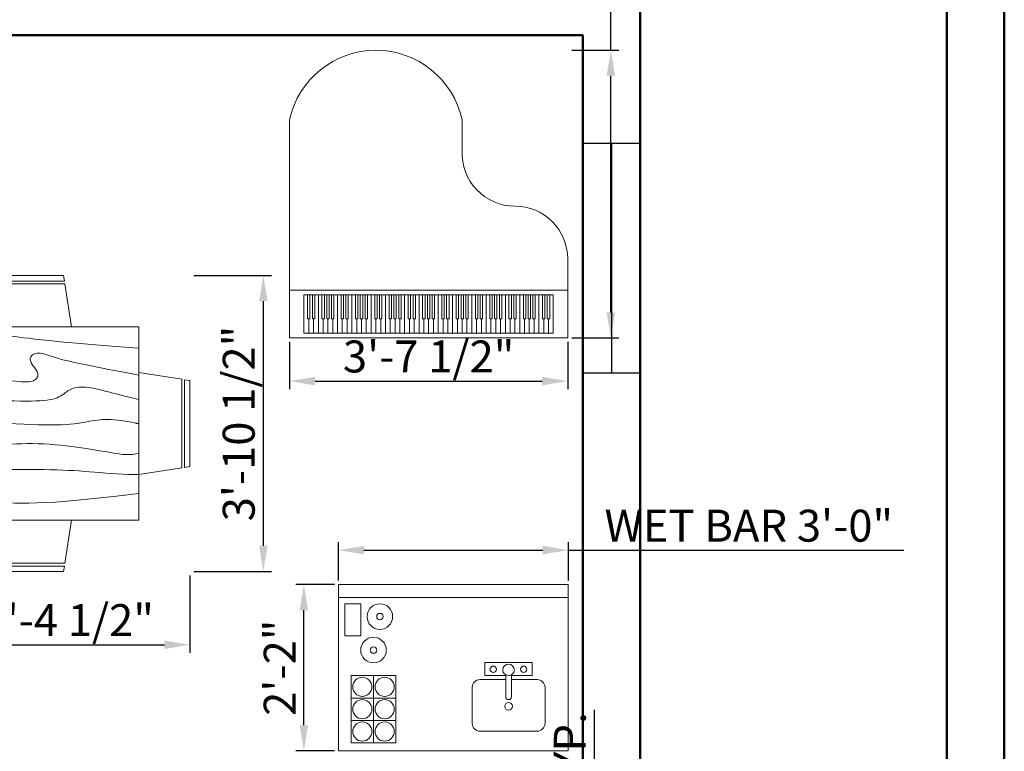
# Model space of a CAD drawing. Units: inches. Extents: x 116541 to 117938, y 135634 to 136328.
# Tile 8 of 9: x 117747 to 117902, y 135965 to 136080. Entities that reach past the tile are written whole.
import ezdxf

# ---------------------------------------------------------------- set-up
doc = ezdxf.new("R2010")
doc.units = ezdxf.units.IN
for name, color, linetype, lineweight in [('A-ANNO-DIMS', 2, 'Continuous', 18), ('A-FURN', 8, 'Continuous', 18), ('A-GLAZ', 1, 'Continuous', 25), ('A-WALL', 7, 'Continuous', 50)]:
    doc.layers.add(name, color=color, linetype=linetype, lineweight=lineweight)
doc.styles.get("Standard").update_dxf_attribs({"font": 'arial.ttf'})
doc.dimstyles.new('ISO-25', dxfattribs={"dimtxt": 5, "dimasz": 4, "dimexe": 1.25, "dimexo": 0.625, "dimtad": 1, "dimdec": 3, "dimlunit": 3, "dimtxsty": 'Standard', "dimcen": 2.5, "dimadec": 0, "dimazin": 0, "dimtfac": 1, "dimtdec": 3, "dimtmove": 0, "dimatfit": 3, "dimfxl": 1, "dimarcsym": 0})

# ---------------------------------------------------------------- blocks, each defined once
blk = doc.blocks.new('Dining Set - 36 x 72 in.')
for p, q in [((-22, 27.5), (-22.1562, 26.50042)), ((-22, 27.5), (-6, 27.5)), ((-5.8437, 26.49966), (-6, 27.5)), ((6, 27.5), (5.8438, 26.50042)), ((6, 27.5), (22, 27.5)), ((22.1563, 26.49966), (22, 27.5)), ((-22.2343, 26.00059), (-23.4847, 17.99762)), ((-22.2304, 26), (-5.7608, 26)), ((-5.8416, 26.5), (-22.1534, 26.5)), ((-4.5152, 17.99762), (-5.7655, 25.99926)), ((5.7657, 26.00059), (4.5153, 17.99762)), ((5.7696, 26), (22.2392, 26)), ((22.1584, 26.5), (5.8466, 26.5)), ((23.4848, 17.99762), (22.2345, 25.99926)), ((36, 18), (-36, 18)), ((-36, 18), (-36, -18)), ((36, -18), (36, 18)), ((-44.0006, 8.23428), (-35.9976, 9.48474)), ((44.0006, 8.23428), (35.9976, 9.48474)), ((-45.5, 8), (-44.5004, 8.15617)), ((-45.5, 8), (-45.5, -8)), ((-44.5, -8.15843), (-44.5, 8.15338)), ((-44, 8.23041), (-44, -8.23915)), ((44, 8.23041), (44, -8.23915)), ((44.5, -8.15843), (44.5, 8.15338)), ((45.5, 8), (44.5005, 8.15617)), ((45.5, 8), (45.5, -8)), ((-44.4997, -8.15631), (-45.5, -8)), ((-35.9976, -9.48476), (-43.9993, -8.2345)), ((35.9976, -9.48476), (43.9993, -8.2345)), ((44.4997, -8.15631), (45.5, -8)), ((-36, -18), (36, -18)), ((-22.2343, -26.0006), (-23.4847, -17.99762)), ((-4.5152, -17.99762), (-5.7655, -25.99928)), ((5.7657, -26.0006), (4.5153, -17.99762)), ((23.4848, -17.99762), (22.2345, -25.99928)), ((-22.2304, -26), (-5.7608, -26)), ((-22, -27.5), (-22.1562, -26.50044)), ((-5.8416, -26.5), (-22.1534, -26.5)), ((-5.8437, -26.49967), (-6, -27.5)), ((5.7696, -26), (22.2392, -26)), ((6, -27.5), (5.8438, -26.50044)), ((22.1584, -26.5), (5.8466, -26.5)), ((22.1563, -26.49967), (22, -27.5)), ((-22, -27.5), (-6, -27.5)), ((6, -27.5), (22, -27.5))]:
    blk.add_line(p, q)
for points in [[(-36, 15), (-31.1772, 14.97754), (-26.8079, 14.91406), (-22.8538, 14.81543), (-19.276, 14.6875), (-16.0362, 14.53613), (-13.0957, 14.36718), (-10.4159, 14.18652), (-7.9583, 14), (-5.6904, 13.81315), (-3.6035, 13.63021), (-1.6954, 13.45508), (0.0365, 13.29166), (1.5945, 13.14388), (2.9811, 13.01562), (4.1988, 12.9108), (5.25, 12.83333), (6.1393, 12.78613), (6.8802, 12.76823), (7.4883, 12.77767), (7.9792, 12.8125), (8.3685, 12.87077), (8.6719, 12.95052), (8.9049, 13.0498), (9.0833, 13.16666), (9.2205, 13.29899), (9.3216, 13.44401), (9.3895, 13.59879), (9.4271, 13.76041), (9.4373, 13.92594), (9.4232, 14.09245), (9.3875, 14.257), (9.3333, 14.41666), (9.2638, 14.56917), (9.1836, 14.71484), (9.0975, 14.85465), (9.0104, 14.98958), (8.9272, 15.1206), (8.8529, 15.2487), (8.7922, 15.37483), (8.75, 15.5), (8.7305, 15.62467), (8.7344, 15.74739), (8.7617, 15.86621), (8.8125, 15.97916), (8.8867, 16.08431), (8.9844, 16.17968), (9.1055, 16.26334), (9.25, 16.33333), (9.4189, 16.38802), (9.6172, 16.42708), (9.8506, 16.45052), (10.125, 16.45833), (10.4463, 16.45052), (10.8203, 16.42708), (11.2529, 16.38802), (11.75, 16.33333), (12.3184, 16.26318), (12.9694, 16.17838), (13.7151, 16.07991), (14.5677, 15.96875), (15.5395, 15.84586), (16.6426, 15.71224), (17.8893, 15.56884), (19.2917, 15.41666), (20.859, 15.25667), (22.5879, 15.08984), (24.4721, 14.91715), (26.5052, 14.73958), (28.6809, 14.5581), (30.9929, 14.3737), (33.4347, 14.18733), (36, 14)], [(-36, 10), (-28.9766, 10.14274), (-23.1725, 10.20442), (-18.4241, 10.19775), (-14.5677, 10.13541), (-11.4399, 10.03011), (-8.877, 9.89453), (-6.7154, 9.74137), (-4.7917, 9.58333), (-2.9698, 9.43082), (-1.2246, 9.28515), (0.4415, 9.14534), (2.026, 9.01041), (3.5266, 8.87939), (4.9408, 8.7513), (6.266, 8.62516), (7.5, 8.5), (8.6411, 8.37549), (9.6914, 8.2539), (10.6538, 8.13818), (11.5312, 8.03125), (12.3267, 7.93603), (13.043, 7.85547), (13.6831, 7.79248), (14.25, 7.75), (14.7471, 7.7303), (15.1797, 7.73307), (15.5537, 7.75732), (15.875, 7.80208), (16.1494, 7.86637), (16.3828, 7.94922), (16.5811, 8.04964), (16.75, 8.16666), (16.8944, 8.29915), (17.0143, 8.44531), (17.1089, 8.60319), (17.1771, 8.77083), (17.218, 8.94629), (17.2305, 9.1276), (17.2137, 9.31282), (17.1667, 9.5), (17.0895, 9.6875), (16.987, 9.875), (16.8649, 10.0625), (16.7292, 10.25), (16.5856, 10.4375), (16.4401, 10.625), (16.2985, 10.8125), (16.1667, 11), (16.05, 11.18733), (15.9518, 11.3737), (15.8752, 11.5581), (15.8229, 11.73958), (15.798, 11.91715), (15.8034, 12.08984), (15.842, 12.25667), (15.9167, 12.41666), (16.0295, 12.56836), (16.1784, 12.70833), (16.3605, 12.83268), (16.5729, 12.9375), (16.8127, 13.01888), (17.0768, 13.07291), (17.3625, 13.0957), (17.6667, 13.08333), (17.9894, 13.03312), (18.3418, 12.94726), (18.7382, 12.82918), (19.1927, 12.68229), (19.7195, 12.51001), (20.3327, 12.31575), (21.0465, 12.10294), (21.875, 11.875), (22.8357, 11.63354), (23.959, 11.37304), (25.2786, 11.08618), (26.8282, 10.76562), (28.6414, 10.40405), (30.752, 9.99414), (33.1936, 9.52856), (36, 9)], [(-36, 5.5), (-30.7157, 5.3348), (-26.069, 5.20963), (-21.9946, 5.11767), (-18.4271, 5.05208), (-15.3009, 5.00602), (-12.5508, 4.97265), (-10.1112, 4.94515), (-7.9167, 4.91666), (-5.909, 4.88167), (-4.0586, 4.83984), (-2.3429, 4.79215), (-0.7396, 4.73958), (0.7739, 4.6831), (2.22, 4.6237), (3.6213, 4.56233), (5, 4.5), (6.373, 4.43782), (7.7344, 4.3776), (9.0723, 4.32129), (10.375, 4.27083), (11.6309, 4.22819), (12.8281, 4.19531), (13.9551, 4.17415), (15, 4.16666), (15.954, 4.17448), (16.819, 4.19791), (17.6001, 4.23698), (18.3021, 4.29166), (18.9299, 4.36198), (19.4883, 4.44791), (19.9823, 4.54948), (20.4167, 4.66666), (20.7969, 4.79899), (21.1302, 4.94401), (21.4245, 5.09879), (21.6875, 5.26041), (21.9271, 5.42594), (22.1511, 5.59245), (22.3672, 5.757), (22.5834, 5.91666), (22.8065, 6.06868), (23.0404, 6.21093), (23.2879, 6.34147), (23.5521, 6.45833), (23.8358, 6.55957), (24.142, 6.64323), (24.4735, 6.70735), (24.8334, 6.75), (25.2235, 6.76969), (25.642, 6.76692), (26.0858, 6.74267), (26.5521, 6.69791), (27.0379, 6.63362), (27.5404, 6.55078), (28.0565, 6.45036), (28.5834, 6.33333), (29.1242, 6.19987), (29.7071, 6.04687), (30.3661, 5.87044), (31.1354, 5.66666), (32.0493, 5.43164), (33.142, 5.16146), (34.4475, 4.85221), (36, 4.5)], [(-36, -1), (-30.7915, -0.6591), (-26.0195, -0.38216), (-21.6519, -0.16284), (-17.6563, 0.00521), (-14.0005, 0.12833), (-10.6523, 0.21289), (-7.5796, 0.26522), (-4.75, 0.29166), (-2.134, 0.29793), (0.2878, 0.28711), (2.5317, 0.26163), (4.6146, 0.22396), (6.5529, 0.17651), (8.3633, 0.12174), (10.0623, 0.06209), (11.6667, 0), (13.1899, -0.06201), (14.6341, -0.1211), (15.9982, -0.17432), (17.2813, -0.21875), (18.4823, -0.25147), (19.6003, -0.26953), (20.6343, -0.27002), (21.5834, -0.25), (22.4481, -0.20768), (23.2357, -0.14584), (23.9549, -0.06836), (24.6146, 0.02083), (25.2235, 0.11784), (25.7904, 0.21875), (26.3241, 0.31966), (26.8334, 0.41666), (27.3265, 0.50618), (27.8099, 0.58593), (28.2894, 0.65397), (28.7709, 0.70833), (29.2601, 0.74707), (29.763, 0.76823), (30.2855, 0.76985), (30.8334, 0.75), (31.4088, 0.70784), (31.9994, 0.64713), (32.589, 0.57275), (33.1615, 0.48958), (33.7008, 0.4025), (34.1908, 0.3164), (34.6153, 0.23616), (34.9584, 0.16666), (35.2099, 0.11165), (35.3848, 0.07031), (35.504, 0.04069), (35.5886, 0.02083), (35.6594, 0.00879), (35.7377, 0.0026), (35.8442, 0.00032), (36, 0)], [(-36, -6.5), (-27.1843, -6.31267), (-20.084, -6.1263), (-14.469, -5.9419), (-10.1094, -5.76042), (-6.7752, -5.58285), (-4.2363, -5.41016), (-2.2629, -5.24333), (-0.625, -5.08334), (0.8708, -4.93099), (2.2715, -4.78646), (3.5872, -4.64974), (4.8281, -4.52084), (6.0046, -4.39974), (7.127, -4.28646), (8.2053, -4.18099), (9.25, -4.08334), (10.2705, -3.99382), (11.2734, -3.91407), (12.2647, -3.84603), (13.25, -3.79167), (14.2354, -3.75293), (15.2266, -3.73177), (16.2295, -3.73015), (17.25, -3.75), (18.2912, -3.79248), (19.3451, -3.85547), (20.4009, -3.93604), (21.4479, -4.03125), (22.4754, -4.13819), (23.4727, -4.25391), (24.4289, -4.37549), (25.3334, -4.5), (26.1785, -4.62492), (26.9694, -4.74935), (27.7145, -4.87281), (28.4219, -4.99479), (29.1, -5.11483), (29.7572, -5.23242), (30.4016, -5.34709), (31.0417, -5.45834), (31.6837, -5.56437), (32.3262, -5.65821), (32.9658, -5.73153), (33.599, -5.77604), (34.2224, -5.78345), (34.8327, -5.74545), (35.4264, -5.65373), (36, -5.5)], [(-36, -10), (-26.4022, -9.81299), (-18.4675, -9.62891), (-11.9839, -9.45069), (-6.7396, -9.28125), (-2.5226, -9.12354), (0.8789, -8.98047), (3.6769, -8.85498), (6.0833, -8.75), (8.2767, -8.66765), (10.3021, -8.60677), (12.1712, -8.56543), (13.8958, -8.54167), (15.4876, -8.53353), (16.9583, -8.53907), (18.3197, -8.55632), (19.5834, -8.58334), (20.7616, -8.61841), (21.8685, -8.66081), (22.9188, -8.71004), (23.9271, -8.76563), (24.9081, -8.82707), (25.8763, -8.89388), (26.8465, -8.96558), (27.8334, -9.04167), (28.8474, -9.12118), (29.8828, -9.20117), (30.93, -9.27824), (31.9792, -9.34896), (33.0205, -9.40991), (34.0443, -9.45768), (35.0407, -9.48885), (36, -9.5)], [(-36, -14.5), (-30.0881, -14.33513), (-25.0332, -14.21224), (-20.7312, -14.12647), (-17.0781, -14.07292), (-13.97, -14.04671), (-11.3027, -14.04297), (-8.9724, -14.05681), (-6.875, -14.08334), (-4.9224, -14.11833), (-3.0905, -14.16016), (-1.3709, -14.20785), (0.2448, -14.26042), (1.7647, -14.3169), (3.1973, -14.3763), (4.5507, -14.43767), (5.8333, -14.5), (7.0554, -14.5621), (8.235, -14.62175), (9.3922, -14.67652), (10.5469, -14.72396), (11.7192, -14.76164), (12.929, -14.78711), (14.1965, -14.79794), (15.5417, -14.79167), (16.9933, -14.76424), (18.6152, -14.70508), (20.4804, -14.60197), (22.6615, -14.44271), (25.2312, -14.21509), (28.2624, -13.9069), (31.8277, -13.50594), (36, -13)]]:
    blk.add_lwpolyline(points)
blk = doc.blocks.new('Piano - Baby Grand')
for p, q in [((-29, 8.250005), (-29, -27.249995)), ((7, 1.250005), (7, 8.250005)), ((29, -20.749995), (29, -27.249995)), ((-29, -27.249995), (-29, -37.249995)), ((29, -27.249995), (-29, -27.249995)), ((-26, -36.249995), (-26, -28.249995)), ((-26, -28.249995), (26, -28.249995)), ((-25.25, -33.249995), (-25.25, -28.249995)), ((-24.75, -28.249995), (-24.75, -33.249995)), ((-24.25, -33.249995), (-24.25, -28.249995)), ((-23.75, -28.249995), (-23.75, -33.249995)), ((-23, -36.249995), (-23, -28.249995)), ((-22.25, -33.249995), (-22.25, -28.249995)), ((-21.75, -28.249995), (-21.75, -33.249995)), ((-21.25, -33.249995), (-21.25, -28.249995)), ((-20.75, -28.249995), (-20.75, -33.249995)), ((-20.25, -33.249995), (-20.25, -28.249995)), ((-19.75, -28.249995), (-19.75, -33.249995)), ((-19, -36.249995), (-19, -28.249995)), ((-18.25, -33.249995), (-18.25, -28.249995)), ((-17.75, -28.249995), (-17.75, -33.249995)), ((-17.25, -33.249995), (-17.25, -28.249995)), ((-16.75, -28.249995), (-16.75, -33.249995)), ((-16, -36.249995), (-16, -28.249995)), ((-15.25, -33.249995), (-15.25, -28.249995)), ((-14.75, -28.249995), (-14.75, -33.249995)), ((-14.25, -33.249995), (-14.25, -28.249995)), ((-13.75, -28.249995), (-13.75, -33.249995)), ((-13.25, -33.249995), (-13.25, -28.249995)), ((-12.75, -28.249995), (-12.75, -33.249995)), ((-12, -36.249995), (-12, -28.249995)), ((-11.25, -33.249995), (-11.25, -28.249995)), ((-10.75, -28.249995), (-10.75, -33.249995)), ((-10.25, -33.249995), (-10.25, -28.249995)), ((-9.75, -28.249995), (-9.75, -33.249995)), ((-9, -36.249995), (-9, -28.249995)), ((-8.25, -33.249995), (-8.25, -28.249995)), ((-7.75, -28.249995), (-7.75, -33.249995)), ((-7.25, -33.249995), (-7.25, -28.249995)), ((-6.75, -28.249995), (-6.75, -33.249995)), ((-6.25, -33.249995), (-6.25, -28.249995)), ((-5.75, -28.249995), (-5.75, -33.249995)), ((-5, -36.249995), (-5, -28.249995)), ((-4.25, -33.249995), (-4.25, -28.249995)), ((-3.75, -28.249995), (-3.75, -33.249995)), ((-3.25, -33.249995), (-3.25, -28.249995)), ((-2.75, -28.249995), (-2.75, -33.249995)), ((-2, -36.249995), (-2, -28.249995)), ((-1.25, -33.249995), (-1.25, -28.249995)), ((-0.75, -28.249995), (-0.75, -33.249995)), ((-0.25, -33.249995), (-0.25, -28.249995)), ((0.25, -28.249995), (0.25, -33.249995)), ((0.75, -33.249995), (0.75, -28.249995)), ((1.25, -28.249995), (1.25, -33.249995)), ((2, -36.249995), (2, -28.249995)), ((2.75, -33.249995), (2.75, -28.249995)), ((3.25, -28.249995), (3.25, -33.249995)), ((3.75, -33.249995), (3.75, -28.249995)), ((4.25, -28.249995), (4.25, -33.249995)), ((5, -36.249995), (5, -28.249995)), ((5.75, -33.249995), (5.75, -28.249995)), ((6.25, -28.249995), (6.25, -33.249995)), ((6.75, -33.249995), (6.75, -28.249995)), ((7.25, -28.249995), (7.25, -33.249995)), ((7.75, -33.249995), (7.75, -28.249995)), ((8.25, -28.249995), (8.25, -33.249995)), ((9, -36.249995), (9, -28.249995)), ((9.75, -33.249995), (9.75, -28.249995)), ((10.25, -28.249995), (10.25, -33.249995)), ((10.75, -33.249995), (10.75, -28.249995)), ((11.25, -28.249995), (11.25, -33.249995)), ((12, -36.249995), (12, -28.249995)), ((12.75, -33.249995), (12.75, -28.249995)), ((13.25, -28.249995), (13.25, -33.249995)), ((13.75, -33.249995), (13.75, -28.249995)), ((14.25, -28.249995), (14.25, -33.249995)), ((14.75, -33.249995), (14.75, -28.249995)), ((15.25, -28.249995), (15.25, -33.249995)), ((16, -36.249995), (16, -28.249995)), ((16.75, -33.249995), (16.75, -28.249995)), ((17.25, -28.249995), (17.25, -33.249995)), ((17.75, -33.249995), (17.75, -28.249995)), ((18.25, -28.249995), (18.25, -33.249995)), ((19, -36.249995), (19, -28.249995)), ((19.75, -33.249995), (19.75, -28.249995)), ((20.25, -28.249995), (20.25, -33.249995)), ((20.75, -33.249995), (20.75, -28.249995)), ((21.25, -28.249995), (21.25, -33.249995)), ((21.75, -33.249995), (21.75, -28.249995)), ((22.25, -28.249995), (22.25, -33.249995)), ((23, -36.249995), (23, -28.249995)), ((23.75, -33.249995), (23.75, -28.249995)), ((24.25, -28.249995), (24.25, -33.249995)), ((24.75, -33.249995), (24.75, -28.249995)), ((25.25, -28.249995), (25.25, -33.249995)), ((26, -36.249995), (26, -28.249995)), ((29, -37.249995), (29, -27.249995)), ((-25, -33.249995), (-25.25, -33.249995)), ((-24.75, -33.249995), (-25, -33.249995)), ((-25, -36.249995), (-25, -33.249995)), ((-24, -33.249995), (-24.25, -33.249995)), ((-23.75, -33.249995), (-24, -33.249995)), ((-24, -36.249995), (-24, -33.249995)), ((-22, -33.249995), (-22.25, -33.249995)), ((-21.75, -33.249995), (-22, -33.249995)), ((-22, -36.249995), (-22, -33.249995)), ((-21, -33.249995), (-21.25, -33.249995)), ((-20.75, -33.249995), (-21, -33.249995)), ((-21, -36.249995), (-21, -33.249995)), ((-20, -33.249995), (-20.25, -33.249995)), ((-19.75, -33.249995), (-20, -33.249995)), ((-20, -36.249995), (-20, -33.249995)), ((-18, -33.249995), (-18.25, -33.249995)), ((-17.75, -33.249995), (-18, -33.249995)), ((-18, -36.249995), (-18, -33.249995)), ((-17, -33.249995), (-17.25, -33.249995)), ((-16.75, -33.249995), (-17, -33.249995)), ((-17, -36.249995), (-17, -33.249995)), ((-15, -33.249995), (-15.25, -33.249995)), ((-14.75, -33.249995), (-15, -33.249995)), ((-15, -36.249995), (-15, -33.249995)), ((-14, -33.249995), (-14.25, -33.249995)), ((-13.75, -33.249995), (-14, -33.249995)), ((-14, -36.249995), (-14, -33.249995)), ((-13, -33.249995), (-13.25, -33.249995)), ((-12.75, -33.249995), (-13, -33.249995)), ((-13, -36.249995), (-13, -33.249995)), ((-11, -33.249995), (-11.25, -33.249995)), ((-10.75, -33.249995), (-11, -33.249995)), ((-11, -36.249995), (-11, -33.249995)), ((-10, -33.249995), (-10.25, -33.249995)), ((-9.75, -33.249995), (-10, -33.249995)), ((-10, -36.249995), (-10, -33.249995)), ((-8, -33.249995), (-8.25, -33.249995)), ((-7.75, -33.249995), (-8, -33.249995)), ((-8, -36.249995), (-8, -33.249995)), ((-7, -33.249995), (-7.25, -33.249995)), ((-6.75, -33.249995), (-7, -33.249995)), ((-7, -36.249995), (-7, -33.249995)), ((-6, -33.249995), (-6.25, -33.249995)), ((-5.75, -33.249995), (-6, -33.249995)), ((-6, -36.249995), (-6, -33.249995)), ((-4, -33.249995), (-4.25, -33.249995)), ((-3.75, -33.249995), (-4, -33.249995)), ((-4, -36.249995), (-4, -33.249995)), ((-3, -33.249995), (-3.25, -33.249995)), ((-2.75, -33.249995), (-3, -33.249995)), ((-3, -36.249995), (-3, -33.249995)), ((-1, -33.249995), (-1.25, -33.249995)), ((-0.75, -33.249995), (-1, -33.249995)), ((-1, -36.249995), (-1, -33.249995)), ((0, -33.249995), (-0.25, -33.249995)), ((0.25, -33.249995), (0, -33.249995)), ((0, -36.249995), (0, -33.249995)), ((1, -33.249995), (0.75, -33.249995)), ((1.25, -33.249995), (1, -33.249995)), ((1, -36.249995), (1, -33.249995)), ((3, -33.249995), (2.75, -33.249995)), ((3.25, -33.249995), (3, -33.249995)), ((3, -36.249995), (3, -33.249995)), ((4, -33.249995), (3.75, -33.249995)), ((4.25, -33.249995), (4, -33.249995)), ((4, -36.249995), (4, -33.249995)), ((6, -33.249995), (5.75, -33.249995)), ((6.25, -33.249995), (6, -33.249995)), ((6, -36.249995), (6, -33.249995)), ((7, -33.249995), (6.75, -33.249995)), ((7.25, -33.249995), (7, -33.249995)), ((7, -36.249995), (7, -33.249995)), ((8, -33.249995), (7.75, -33.249995)), ((8.25, -33.249995), (8, -33.249995)), ((8, -36.249995), (8, -33.249995)), ((10, -33.249995), (9.75, -33.249995)), ((10.25, -33.249995), (10, -33.249995)), ((10, -36.249995), (10, -33.249995)), ((11, -33.249995), (10.75, -33.249995)), ((11.25, -33.249995), (11, -33.249995)), ((11, -36.249995), (11, -33.249995)), ((13, -33.249995), (12.75, -33.249995)), ((13.25, -33.249995), (13, -33.249995)), ((13, -36.249995), (13, -33.249995)), ((14, -33.249995), (13.75, -33.249995)), ((14.25, -33.249995), (14, -33.249995)), ((14, -36.249995), (14, -33.249995)), ((15, -33.249995), (14.75, -33.249995)), ((15.25, -33.249995), (15, -33.249995)), ((15, -36.249995), (15, -33.249995)), ((17, -33.249995), (16.75, -33.249995)), ((17.25, -33.249995), (17, -33.249995)), ((17, -36.249995), (17, -33.249995)), ((18, -33.249995), (17.75, -33.249995)), ((18.25, -33.249995), (18, -33.249995)), ((18, -36.249995), (18, -33.249995)), ((20, -33.249995), (19.75, -33.249995)), ((20.25, -33.249995), (20, -33.249995)), ((20, -36.249995), (20, -33.249995)), ((21, -33.249995), (20.75, -33.249995)), ((21.25, -33.249995), (21, -33.249995)), ((21, -36.249995), (21, -33.249995)), ((22, -33.249995), (21.75, -33.249995)), ((22.25, -33.249995), (22, -33.249995)), ((22, -36.249995), (22, -33.249995)), ((24, -33.249995), (23.75, -33.249995)), ((24.25, -33.249995), (24, -33.249995)), ((24, -36.249995), (24, -33.249995)), ((25, -33.249995), (24.75, -33.249995)), ((25.25, -33.249995), (25, -33.249995)), ((25, -36.249995), (25, -33.249995)), ((-26, -36.249995), (-25, -36.249995)), ((-25, -36.249995), (-24, -36.249995)), ((-24, -36.249995), (-23, -36.249995)), ((-23, -36.249995), (-22, -36.249995)), ((-22, -36.249995), (-21, -36.249995)), ((-21, -36.249995), (-20, -36.249995)), ((-20, -36.249995), (-19, -36.249995)), ((-19, -36.249995), (-18, -36.249995)), ((-18, -36.249995), (-17, -36.249995)), ((-17, -36.249995), (-16, -36.249995)), ((-16, -36.249995), (-15, -36.249995)), ((-15, -36.249995), (-14, -36.249995)), ((-14, -36.249995), (-13, -36.249995)), ((-13, -36.249995), (-12, -36.249995)), ((-12, -36.249995), (-11, -36.249995)), ((-11, -36.249995), (-10, -36.249995)), ((-10, -36.249995), (-9, -36.249995)), ((-9, -36.249995), (-8, -36.249995)), ((-8, -36.249995), (-7, -36.249995)), ((-7, -36.249995), (-6, -36.249995)), ((-6, -36.249995), (-5, -36.249995)), ((-5, -36.249995), (-4, -36.249995)), ((-4, -36.249995), (-3, -36.249995)), ((-3, -36.249995), (-2, -36.249995)), ((-2, -36.249995), (-1, -36.249995)), ((-1, -36.249995), (0, -36.249995)), ((0, -36.249995), (1, -36.249995)), ((1, -36.249995), (2, -36.249995)), ((2, -36.249995), (3, -36.249995)), ((3, -36.249995), (4, -36.249995)), ((4, -36.249995), (5, -36.249995)), ((5, -36.249995), (6, -36.249995)), ((6, -36.249995), (7, -36.249995)), ((7, -36.249995), (8, -36.249995)), ((8, -36.249995), (9, -36.249995)), ((9, -36.249995), (10, -36.249995)), ((10, -36.249995), (11, -36.249995)), ((11, -36.249995), (12, -36.249995)), ((12, -36.249995), (13, -36.249995)), ((13, -36.249995), (14, -36.249995)), ((14, -36.249995), (15, -36.249995)), ((15, -36.249995), (16, -36.249995)), ((16, -36.249995), (17, -36.249995)), ((17, -36.249995), (18, -36.249995)), ((18, -36.249995), (19, -36.249995)), ((19, -36.249995), (20, -36.249995)), ((20, -36.249995), (21, -36.249995)), ((21, -36.249995), (22, -36.249995)), ((22, -36.249995), (23, -36.249995)), ((23, -36.249995), (24, -36.249995)), ((24, -36.249995), (25, -36.249995)), ((25, -36.249995), (26, -36.249995)), ((-29, -37.249995), (29, -37.249995))]:
    blk.add_line(p, q)
for centre, radius, start, end in [((-11, 4.327585), 18.42241, 12.29325, 167.7067), ((18, 1.250005), 11, 177.3974, 270), ((18, -20.749995), 11, 0, 90)]:
    blk.add_arc(centre, radius, start, end)
blk = doc.blocks.new('Wet Bar')
for p, q in [((0, 0), (36, 0)), ((0, -26), (0, 0)), ((36, 0), (36, -26)), ((0, -2), (36, -2)), ((3.5, -3), (1, -3)), ((1, -3), (1, -8)), ((3.5, -8), (3.5, -3)), ((1, -8), (3.5, -8)), ((2, -14.25), (9, -14.25)), ((2, -24.75), (2, -14.25)), ((5.5, -14.25), (5.5, -24.75)), ((9, -14.25), (9, -24.75)), ((26.2, -17.55), (26.2, -14.1284)), ((27.1001, -17.55), (27.1001, -14.1284)), ((2, -17.75), (9, -17.75)), ((9, -21.25), (2, -21.25)), ((36, -26), (0, -26)), ((9, -24.75), (2, -24.75))]:
    blk.add_line(p, q)
for points in [[(26.2, -14.25), (22.95, -14.25), (22.95, -12.2), (26.75, -12.2)], [(26.7487, -12.2), (30.3501, -12.2), (30.3501, -14.25), (27.1001, -14.25)], [(22.15, -14.85), (26.2, -14.85)], [(27.1001, -14.85), (31.15, -14.85)], [(20.95, -21.75), (20.95, -16.05)], [(32.3501, -16.05), (32.3501, -21.75)], [(31.15, -22.95), (22.15, -22.95)]]:
    blk.add_lwpolyline(points)
for centre, radius in [((6.5, -5), 2), ((6.5, -5), 0.5), ((5.5, -10.25), 2), ((5.5, -10.25), 0.5), ((24.25, -13.25), 0.5), ((26.65, -13.35), 0.9), ((29, -13.25), 0.5), ((3.75, -16), 1.5), ((7.25, -16), 1.5), ((3.75, -19.5), 1.5), ((7.25, -19.5), 1.5), ((26.65, -19.05), 0.6), ((3.75, -23), 1.5), ((7.25, -23), 1.5)]:
    blk.add_circle(centre, radius)
for centre, radius, start, end in [((22.2251, -16.125), 1.2772, 93.36646, 176.6335), ((31.075, -16.125), 1.2772, 3.366461, 86.63354), ((26.65, -17.55), 0.45, 180, 0), ((22.2251, -21.675), 1.2772, 183.3665, 266.6335), ((31.075, -21.675), 1.2772, 273.3665, 356.6335)]:
    blk.add_arc(centre, radius, start, end)
blk = doc.blocks.new('*D61')
at = {"layer": 'A-ANNO-DIMS', "color": 0, "lineweight": -2, "transparency": 16777216}
for p, q in [((117837.36, 135924.99), (117837.36, 135971.9)), ((117835.14, 135924.99), (117838.61, 135924.99)), ((117837.36, 135913.66), (117837.36, 135920.99)), ((117835.14, 135909.66), (117838.61, 135909.66))]:
    blk.add_line(p, q, dxfattribs=at)
at = {"layer": 'A-ANNO-DIMS', "color": 0, "transparency": 16777216}
for points in [[(117836.7, 135920.99), (117838.03, 135920.99), (117837.36, 135924.99)], [(117836.7, 135913.66), (117838.03, 135913.66), (117837.36, 135909.66)]]:
    blk.add_solid(points, dxfattribs=at)
at = {"layer": 'Defpoints', "color": 0, "transparency": 16777216}
for p in [(117834.51, 135924.99), (117837.36, 135924.99), (117834.51, 135909.66)]:
    blk.add_point(p, dxfattribs=at)
at = {"layer": 'A-ANNO-DIMS', "color": 0, "transparency": 16777216, "insert": (117834.15, 135950.44), "char_height": 5, "attachment_point": 5, "rotation": 90}
blk.add_mtext('1\'-3 1/2" TYP.', dxfattribs=at)
blk = doc.blocks.new('*D80')
at = {"layer": 'A-ANNO-DIMS', "color": 0, "lineweight": -2, "transparency": 16777216}
for p, q in [((117697.46, 135992.95), (117697.46, 135980.84)), ((117774.05, 135992.95), (117774.05, 135980.84)), ((117701.46, 135982.09), (117770.05, 135982.09))]:
    blk.add_line(p, q, dxfattribs=at)
at = {"layer": 'A-ANNO-DIMS', "color": 0, "transparency": 16777216}
for points in [[(117701.46, 135982.75), (117701.46, 135981.42), (117697.46, 135982.09)], [(117770.05, 135982.75), (117770.05, 135981.42), (117774.05, 135982.09)]]:
    blk.add_solid(points, dxfattribs=at)
at = {"layer": 'Defpoints', "color": 0, "transparency": 16777216}
for p in [(117697.46, 135993.58), (117774.05, 135993.58), (117774.05, 135982.09)]:
    blk.add_point(p, dxfattribs=at)
at = {"layer": 'A-ANNO-DIMS', "color": 0, "transparency": 16777216, "insert": (117735.75, 135985.3), "char_height": 5, "attachment_point": 5}
blk.add_mtext('DINING SET 6\'-4 1/2"', dxfattribs=at)
blk = doc.blocks.new('*D81')
at = {"layer": 'A-ANNO-DIMS', "color": 0, "lineweight": -2, "transparency": 16777216}
for p, q in [((117774.67, 136039.87), (117786.79, 136039.87)), ((117785.54, 135997.58), (117785.54, 136035.87)), ((117774.67, 135993.58), (117786.79, 135993.58))]:
    blk.add_line(p, q, dxfattribs=at)
at = {"layer": 'A-ANNO-DIMS', "color": 0, "transparency": 16777216}
for points in [[(117784.87, 136035.87), (117786.2, 136035.87), (117785.54, 136039.87)], [(117784.87, 135997.58), (117786.2, 135997.58), (117785.54, 135993.58)]]:
    blk.add_solid(points, dxfattribs=at)
at = {"layer": 'Defpoints', "color": 0, "transparency": 16777216}
for p in [(117774.05, 136039.87), (117785.54, 136039.87), (117774.05, 135993.58)]:
    blk.add_point(p, dxfattribs=at)
at = {"layer": 'A-ANNO-DIMS', "color": 0, "transparency": 16777216, "insert": (117782.33, 136016.72), "char_height": 5, "attachment_point": 5, "rotation": 90}
blk.add_mtext('3\'-10 1/2"', dxfattribs=at)
blk = doc.blocks.new('*D96')
at = {"layer": 'A-ANNO-DIMS', "color": 0, "lineweight": -2, "transparency": 16777216}
for p, q in [((117839.93, 136075.15), (117839.93, 136164.88)), ((117833.8, 136075.15), (117841.18, 136075.15)), ((117839.93, 136034.11), (117839.93, 136071.15)), ((117833.8, 136030.11), (117841.18, 136030.11))]:
    blk.add_line(p, q, dxfattribs=at)
at = {"layer": 'A-ANNO-DIMS', "color": 0, "transparency": 16777216}
for points in [[(117839.26, 136071.15), (117840.6, 136071.15), (117839.93, 136075.15)], [(117839.26, 136034.11), (117840.6, 136034.11), (117839.93, 136030.11)]]:
    blk.add_solid(points, dxfattribs=at)
at = {"layer": 'Defpoints', "color": 0, "transparency": 16777216}
for p in [(117833.18, 136075.15), (117839.93, 136075.15), (117833.18, 136030.11)]:
    blk.add_point(p, dxfattribs=at)
at = {"layer": 'A-ANNO-DIMS', "color": 0, "transparency": 16777216, "insert": (117836.72, 136122.01), "char_height": 5, "attachment_point": 5, "rotation": 90}
blk.add_mtext('BABY GRAND PIANO 3\'-9"', dxfattribs=at)
blk = doc.blocks.new('*D97')
at = {"layer": 'A-ANNO-DIMS', "color": 0, "lineweight": -2, "transparency": 16777216}
for p, q in [((117789.64, 136029.49), (117789.64, 136022.11)), ((117833.18, 136029.49), (117833.18, 136022.11)), ((117793.64, 136023.36), (117829.18, 136023.36))]:
    blk.add_line(p, q, dxfattribs=at)
at = {"layer": 'A-ANNO-DIMS', "color": 0, "transparency": 16777216}
for points in [[(117793.64, 136024.02), (117793.64, 136022.69), (117789.64, 136023.36)], [(117829.18, 136024.02), (117829.18, 136022.69), (117833.18, 136023.36)]]:
    blk.add_solid(points, dxfattribs=at)
at = {"layer": 'Defpoints', "color": 0, "transparency": 16777216}
for p in [(117789.64, 136030.11), (117833.18, 136030.11), (117833.18, 136023.36)]:
    blk.add_point(p, dxfattribs=at)
at = {"layer": 'A-ANNO-DIMS', "color": 0, "transparency": 16777216, "insert": (117811.41, 136026.57), "char_height": 5, "attachment_point": 5}
blk.add_mtext('3\'-7 1/2"', dxfattribs=at)
blk = doc.blocks.new('*D98')
at = {"layer": 'A-ANNO-DIMS', "color": 0, "lineweight": -2, "transparency": 16777216}
for p, q in [((117797.28, 135992.13), (117797.28, 135998.15)), ((117833.28, 135992.13), (117833.28, 135998.15)), ((117801.28, 135996.9), (117829.28, 135996.9)), ((117833.28, 135996.9), (117885.78, 135996.9))]:
    blk.add_line(p, q, dxfattribs=at)
at = {"layer": 'A-ANNO-DIMS', "color": 0, "transparency": 16777216}
for points in [[(117801.28, 135997.57), (117801.28, 135996.24), (117797.28, 135996.9)], [(117829.28, 135997.57), (117829.28, 135996.24), (117833.28, 135996.9)]]:
    blk.add_solid(points, dxfattribs=at)
at = {"layer": 'Defpoints', "color": 0, "transparency": 16777216}
for p in [(117833.28, 135996.9), (117797.28, 135991.5), (117833.28, 135991.5)]:
    blk.add_point(p, dxfattribs=at)
at = {"layer": 'A-ANNO-DIMS', "color": 0, "transparency": 16777216, "insert": (117861.53, 136000.08), "char_height": 5, "attachment_point": 5}
blk.add_mtext('WET BAR 3\'-0"', dxfattribs=at)
blk = doc.blocks.new('*D99')
at = {"layer": 'A-ANNO-DIMS', "color": 0, "lineweight": -2, "transparency": 16777216}
for p, q in [((117796.65, 135991.5), (117790.63, 135991.5)), ((117791.88, 135969.5), (117791.88, 135987.5)), ((117796.65, 135965.5), (117790.63, 135965.5))]:
    blk.add_line(p, q, dxfattribs=at)
at = {"layer": 'A-ANNO-DIMS', "color": 0, "transparency": 16777216}
for points in [[(117791.21, 135987.5), (117792.54, 135987.5), (117791.88, 135991.5)], [(117791.21, 135969.5), (117792.54, 135969.5), (117791.88, 135965.5)]]:
    blk.add_solid(points, dxfattribs=at)
at = {"layer": 'Defpoints', "color": 0, "transparency": 16777216}
for p in [(117791.88, 135991.5), (117797.28, 135991.5), (117797.28, 135965.5)]:
    blk.add_point(p, dxfattribs=at)
at = {"layer": 'A-ANNO-DIMS', "color": 0, "transparency": 16777216, "insert": (117788.74, 135978.5), "char_height": 5, "attachment_point": 5, "rotation": 90}
blk.add_mtext('2\'-2"', dxfattribs=at)

msp = doc.modelspace()

# ---------------------------------------------------------------- linework, layer by layer
at = {"layer": 'A-GLAZ'}
msp.add_line((117840.0209, 136060.6013), (117840.0209, 136024.6013), dxfattribs=at)
msp.add_lwpolyline([(117835.5209, 136060.6013), (117844.5209, 136060.6013), (117844.5209, 136024.6013), (117835.5209, 136024.6013)], close=True, dxfattribs=at)
at = {"layer": 'A-WALL'}
for p, q in [((117901.5209, 136286.5034), (117901.5209, 135734.5034)), ((117844.5209, 135951.0034), (117844.5209, 136253.5034)), ((117892.5209, 136244.5034), (117892.5209, 135750.0323)), ((117835.5209, 136077.5034), (117697.9632, 136077.5034)), ((117835.5209, 135956.0034), (117835.5209, 136077.5034))]:
    msp.add_line(p, q, dxfattribs=at)

# ---------------------------------------------------------------- block references
at = {"layer": 'A-FURN'}
for name, p, xscale, yscale, zscale in [('Piano - Baby Grand', (117811.4102, 136058.0701), 0.7505533916438766, 0.7505533916438766, 0.7505533916438766), ('Dining Set - 36 x 72 in.', (117735.7537, 136016.7204), 0.8416470728042412, 0.8416470728042412, 0.8416470728042412)]:
    msp.add_blockref(name, p, dxfattribs=dict(at, xscale=xscale, yscale=yscale, zscale=zscale))
msp.add_blockref('Wet Bar', (117797.2764, 135991.5047), dxfattribs=at)

# ---------------------------------------------------------------- dimensions: what is measured, and where the dimension line sits
at = {"layer": 'A-ANNO-DIMS'}
for base, p1, p2, text, picture, middle in [((117839.9312, 136075.1452), (117833.1762, 136030.112), (117833.1762, 136075.1452), 'BABY GRAND PIANO <>', '*D96', (117836.7175, 136122.0144)), ((117837.365, 135924.9875), (117834.5148, 135909.6557), (117834.5148, 135924.9875), '<> TYP.', '*D61', (117834.153, 135950.4413))]:
    dim = msp.add_linear_dim(base=base, p1=p1, p2=p2, angle=90, text=text, dimstyle='ISO-25', override={"dimdec": 1, "dimrnd": 0, "dimzin": 1, "dimlunit": 4, "dimfrac": 2}, dxfattribs=at)
    dim.commit()
    dim.dimension.update_dxf_attribs({"geometry": picture, "text_midpoint": middle})
for base, p1, p2, picture, middle in [((117785.5371, 136039.8657), (117774.0487, 135993.5751), (117774.0487, 136039.8657), '*D81', (117782.3252, 136016.7204)), ((117791.8764, 135991.5047), (117797.2764, 135965.5047), (117797.2764, 135991.5047), '*D99', (117788.7412, 135978.5047))]:
    dim = msp.add_linear_dim(base=base, p1=p1, p2=p2, angle=90, dimstyle='ISO-25', override={"dimdec": 1, "dimrnd": 0, "dimzin": 1, "dimlunit": 4, "dimfrac": 2}, dxfattribs=at)
    dim.commit()
    dim.dimension.update_dxf_attribs({"geometry": picture, "text_midpoint": middle})
dim = msp.add_linear_dim(base=(117833.1762, 136023.357), p1=(117789.6441, 136030.112), p2=(117833.1762, 136030.112), dimstyle='ISO-25', override={"dimdec": 1, "dimrnd": 0, "dimzin": 1, "dimlunit": 4, "dimfrac": 2}, dxfattribs=at)
dim.commit()
dim.dimension.update_dxf_attribs({"geometry": '*D97', "text_midpoint": (117811.4102, 136026.5689)})
for base, p1, p2, text, picture, middle in [((117833.2764, 135996.9047), (117797.2764, 135991.5047), (117833.2764, 135991.5047), 'WET BAR <>', '*D98', (117861.5303, 136000.0842)), ((117774.0487, 135982.0866), (117697.4588, 135993.5751), (117774.0487, 135993.5751), 'DINING SET <>', '*D80', (117735.7537, 135985.2969))]:
    dim = msp.add_linear_dim(base=base, p1=p1, p2=p2, text=text, dimstyle='ISO-25', override={"dimdec": 1, "dimrnd": 0, "dimzin": 1, "dimlunit": 4, "dimfrac": 2}, dxfattribs=at)
    dim.commit()
    dim.dimension.update_dxf_attribs({"geometry": picture, "text_midpoint": middle})

doc.saveas('drawing.dxf')
